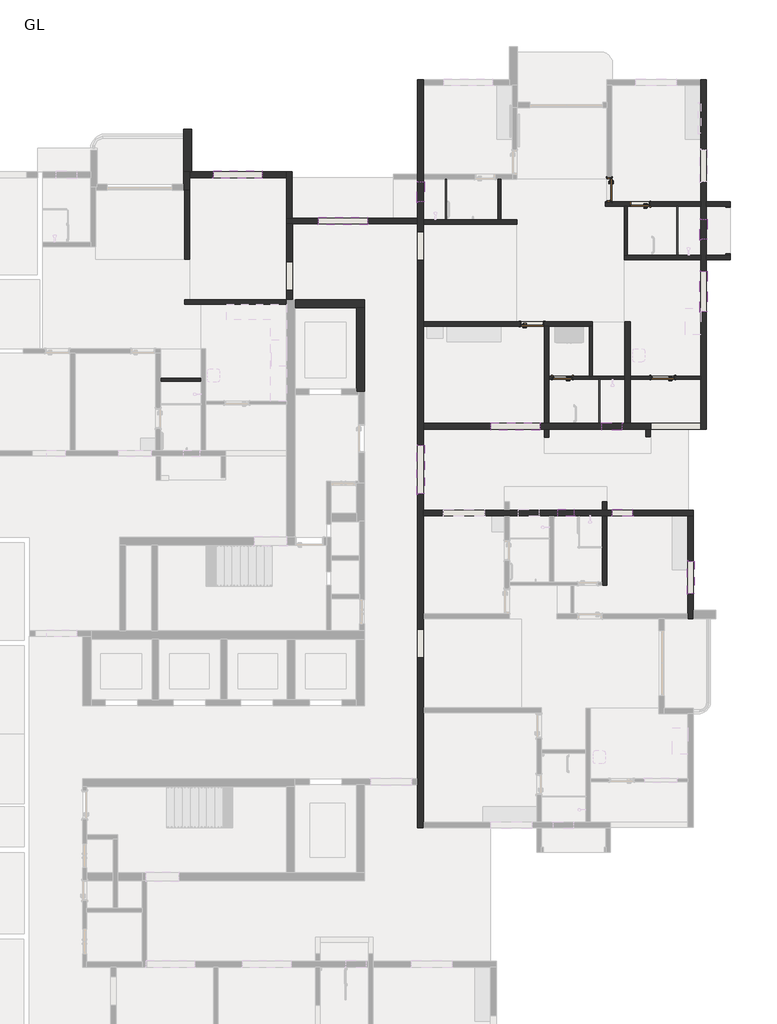
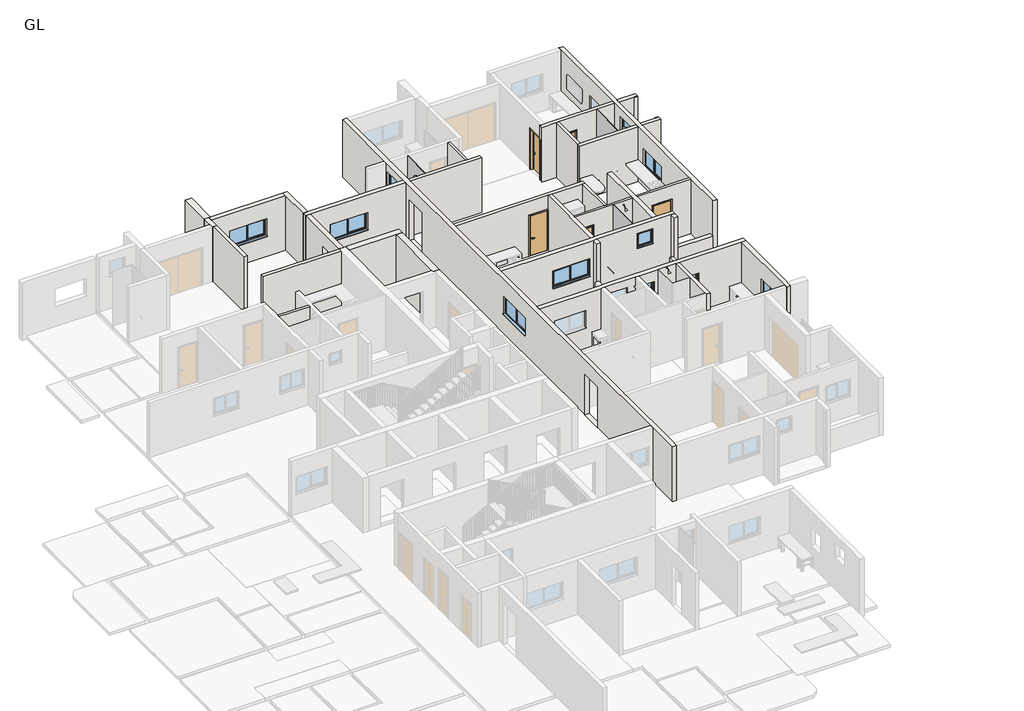
# One storey, part 6 of 14: 34 walls, 11 windows, 5 doors, 3 plates.
"""IFC4 building model written with IfcOpenShell, lengths in millimetres."""

from ifc_helpers import new_model, si_unit, origin, origin_with_axes, place, context, project, spatial, polyline, outline, extrude, faceted_brep, transform, mapped, element, save
from components import doors_intsgl_2_5_door_21b53886, doors_intsgl_2_5_door_ce04bd24, doors_intsgl_3_door_8261d8fb, doors_intsgl_3_door_f61d7fb9, doors_intsgl_3_door_77e94e6e, system_panel_glazed_1e7c63f8, system_panel_glazed_6ac8334b, system_panel_glazed_da641326, windows_dbl_plain_2_5_f94f9a84, windows_dbl_plain_4_905afcad, windows_dbl_plain_5_907a13a5, windows_dbl_plain_6_3da2432f, windows_sgl_plain_2_298b83e7, windows_sgl_plain_2_5_21186da1

model = new_model("IFC4")

# Units and contexts
model_context = context("Model", 3, world=origin())
ifc_project = project(units=[si_unit("LENGTHUNIT", "METRE", prefix="MILLI")], contexts=[model_context])

# Site, building, storey
site = spatial("IfcSite", under=ifc_project)
building = spatial("IfcBuilding", under=site)
storey = spatial("IfcBuildingStorey", under=building, Name="GL", Elevation=0.0)

# Doors
placement = place(None, origin())
doors_intsgl_2_5_door_shape = doors_intsgl_2_5_door_21b53886(model_context)
element("IfcDoor", 1, ObjectType="Doors_IntSgl : 2.5' DOOR", at=placement, inside=storey, context=model_context, shape_type="MappedRepresentation", body=[
    mapped(doors_intsgl_2_5_door_shape, transform((14743.1475488, 88467.3437403, 149.9616), x_axis=(-1.0, 0.0, 0.0), y_axis=(0.0, -1.0, 0.0), z_axis=(0.0, 0.0, 1.0))),
])
doors_intsgl_2_5_door_2_shape = doors_intsgl_2_5_door_ce04bd24(model_context)
element("IfcDoor", 2, ObjectType="Doors_IntSgl : 2.5' DOOR", at=placement, inside=storey, context=model_context, shape_type="MappedRepresentation", body=[
    mapped(doors_intsgl_2_5_door_2_shape, transform((17655.4725595, 94980.9320056, 149.9616), x_axis=(-1.0, 0.0, 0.0), y_axis=(0.0, -1.0, 0.0), z_axis=(0.0, 0.0, 1.0))),
])
doors_intsgl_3_door_shape = doors_intsgl_3_door_8261d8fb(model_context)
element("IfcDoor", 3, ObjectType="Doors_IntSgl : 3' DOOR", at=placement, inside=storey, context=model_context, shape_type="MappedRepresentation", body=[
    mapped(doors_intsgl_3_door_shape, transform((13604.2115488, 90484.8048694, 149.9616), x_axis=(1.0, 0.0, 0.0), y_axis=(0.0, 1.0, 0.0), z_axis=(0.0, 0.0, 1.0))),
])
doors_intsgl_3_door_2_shape = doors_intsgl_3_door_f61d7fb9(model_context)
element("IfcDoor", 4, ObjectType="Doors_IntSgl : 3' DOOR", at=placement, inside=storey, context=model_context, shape_type="MappedRepresentation", body=[
    mapped(doors_intsgl_3_door_2_shape, transform((16503.5076703, 95525.0000056, 149.9616), x_axis=(0.0, -1.0, 0.0), y_axis=(1.0, 0.0, 0.0), z_axis=(0.0, 0.0, 1.0))),
])
doors_intsgl_3_door_3_shape = doors_intsgl_3_door_77e94e6e(model_context)
element("IfcDoor", 5, ObjectType="Doors_IntSgl : 3' DOOR", at=placement, inside=storey, context=model_context, shape_type="MappedRepresentation", body=[
    mapped(doors_intsgl_3_door_3_shape, transform((18512.1396703, 88467.3437403, 149.9616), x_axis=(-1.0, 0.0, 0.0), y_axis=(0.0, -1.0, 0.0), z_axis=(0.0, 0.0, 1.0))),
])

# Plates
system_panel_glazed_shape = system_panel_glazed_1e7c63f8(model_context)
element("IfcPlate", 6, ObjectType="System Panel : Glazed", at=placement, inside=storey, context=model_context, shape_type="MappedRepresentation", body=[
    mapped(system_panel_glazed_shape, transform((16166.2969726, 87590.005818, 0.0), x_axis=(0.0, 1.0, 0.0), y_axis=(-1.0, 0.0, 0.0), z_axis=(0.0, 0.0, 1.0))),
])
system_panel_glazed_2_shape = system_panel_glazed_6ac8334b(model_context)
element("IfcPlate", 7, ObjectType="System Panel : Glazed", at=placement, inside=storey, context=model_context, shape_type="MappedRepresentation", body=[
    mapped(system_panel_glazed_2_shape, transform((19020.1396703, 93980.8602696, 0.0), x_axis=(0.0, -1.0, 0.0), y_axis=(1.0, 0.0, 0.0), z_axis=(0.0, 0.0, 1.0))),
])
system_panel_glazed_3_shape = system_panel_glazed_da641326(model_context)
element("IfcPlate", 8, ObjectType="System Panel : Glazed", at=placement, inside=storey, context=model_context, shape_type="MappedRepresentation", body=[
    mapped(system_panel_glazed_3_shape, transform((10397.1569726, 95164.1635363, 0.0), x_axis=(0.0, 1.0, 0.0), y_axis=(-1.0, 0.0, 0.0), z_axis=(0.0, 0.0, 1.0))),
])

# Walls
element("IfcWall", 9, ObjectType="W2", at=placement, inside=storey, context=model_context, shape_type="Brep", body=[
    faceted_brep([(16231.9624579, 83273.9078957, 0.0), (16231.9624579, 80772.0078957, 0.0), (16231.9624579, 80657.7078957, 0.0), (16231.9624579, 80657.7078957, 3000.0), (16231.9624579, 80772.0078957, 3000.0), (16231.9624579, 83273.9078957, 3000.0), (16405.6984579, 83273.9078957, 0.0), (16405.6984579, 83273.9078957, 3000.0), (16405.6984579, 80657.7078957, 3000.0), (16405.6984579, 80657.7078957, 0.0)], [[[0, 1, 2, 3, 4, 5]], [[6, 7, 8, 9]], [[2, 1, 0, 6, 9]], [[5, 4, 3, 8, 7]], [[0, 5, 7, 6]], [[3, 2, 9, 8]]]),
])
element("IfcWall", 10, ObjectType="W2", at=placement, inside=storey, context=model_context, shape_type="Brep", body=[
    faceted_brep([(17071.2725595, 93067.6565337, 0.0), (17071.2725595, 93067.6565337, 3000.0), (17185.5725595, 93067.6565337, 3000.0), (19934.5396703, 93067.6565337, 3000.0), (19934.5396703, 93067.6565337, 0.0), (17185.5725595, 93067.6565337, 0.0), (17071.2725595, 92893.9205337, 3000.0), (17071.2725595, 92893.9205337, 0.0), (19934.5396703, 92893.9205337, 0.0), (19934.5396703, 92893.9205337, 3000.0)], [[[0, 1, 2, 3, 4, 5]], [[6, 7, 8, 9]], [[7, 0, 5, 4, 8]], [[1, 6, 9, 3, 2]], [[4, 3, 9, 8]], [[1, 0, 7, 6]]]),
    faceted_brep([(21055.8975595, 93067.6565337, 3000.0), (21055.8975595, 93067.6565337, 0.0), (20882.1615595, 93067.6565337, 0.0), (20147.8996703, 93067.6565337, 0.0), (20147.8996703, 93067.6565337, 3000.0), (20882.1615595, 93067.6565337, 3000.0), (21055.8975595, 92893.9205337, 0.0), (21055.8975595, 92893.9205337, 3000.0), (20147.8996703, 92893.9205337, 3000.0), (20147.8996703, 92893.9205337, 0.0)], [[[0, 1, 2, 3, 4, 5]], [[6, 7, 8, 9]], [[1, 6, 9, 3, 2]], [[7, 0, 5, 4, 8]], [[4, 3, 9, 8]], [[1, 0, 7, 6]]]),
])
element("IfcWall", 11, ObjectType="W2", at=placement, inside=storey, context=model_context, shape_type="Brep", body=[
    faceted_brep([(16360.0725595, 95067.8000056, 0.0), (16360.0725595, 95067.8000056, 3000.0), (16416.6396703, 95067.8000056, 3000.0), (16590.3756703, 95067.8000056, 3000.0), (19934.5396703, 95067.8000056, 3000.0), (19934.5396703, 95067.8000056, 0.0), (16590.3756703, 95067.8000056, 0.0), (16416.6396703, 95067.8000056, 0.0), (17274.4725595, 95067.8000056, 2259.9616), (17274.4725595, 95067.8000056, 149.9616), (18036.4725595, 95067.8000056, 149.9616), (18036.4725595, 95067.8000056, 2259.9616), (16360.0725595, 94894.0640056, 3000.0), (16360.0725595, 94894.0640056, 0.0), (17071.2725595, 94894.0640056, 0.0), (17185.5725595, 94894.0640056, 0.0), (19934.5396703, 94894.0640056, 0.0), (19934.5396703, 94894.0640056, 3000.0), (17185.5725595, 94894.0640056, 3000.0), (17071.2725595, 94894.0640056, 3000.0), (17274.4725595, 94894.0640056, 149.9616), (17274.4725595, 94894.0640056, 2259.9616), (18036.4725595, 94894.0640056, 2259.9616), (18036.4725595, 94894.0640056, 149.9616)], [[[0, 1, 2, 3, 4, 5, 6, 7], [8, 9, 10, 11]], [[12, 13, 14, 15, 16, 17, 18, 19], [20, 21, 22, 23]], [[13, 0, 7, 6, 5, 16, 15, 14]], [[1, 0, 13, 12]], [[1, 12, 19, 18, 17, 4, 3, 2]], [[5, 4, 17, 16]], [[20, 9, 8, 21]], [[21, 8, 11, 22]], [[10, 23, 22, 11]], [[9, 20, 23, 10]]]),
    faceted_brep([(21055.8975595, 95067.8000056, 3000.0), (21055.8975595, 95067.8000056, 0.0), (20147.8996703, 95067.8000056, 0.0), (20147.8996703, 95067.8000056, 3000.0), (21055.8975595, 94894.0640056, 0.0), (21055.8975595, 94894.0640056, 3000.0), (20882.1615595, 94894.0640056, 3000.0), (20147.8996703, 94894.0640056, 3000.0), (20147.8996703, 94894.0640056, 0.0), (20882.1615595, 94894.0640056, 0.0)], [[[0, 1, 2, 3]], [[4, 5, 6, 7, 8, 9]], [[1, 4, 9, 8, 2]], [[5, 0, 3, 7, 6]], [[3, 2, 8, 7]], [[1, 0, 5, 4]]]),
])
element("IfcWall", 12, ObjectType="W2", at=placement, inside=storey, context=model_context, shape_type="SweptSolid", body=[
    extrude(outline(polyline([(20882.1615595, 94855.9640056), (20882.1615595, 94894.0640056), (21055.8975595, 94894.0640056), (21055.8975595, 94855.9640056), (20882.1615595, 94855.9640056)])), origin_with_axes(), (0.0, 0.0, 1.0), 3000.0),
])
element("IfcWall", 13, ObjectType="W2", at=placement, inside=storey, context=model_context, shape_type="SweptSolid", body=[
    extrude(outline(polyline([(20882.1615595, 93067.6565337), (20882.1615595, 93112.1065337), (21055.8975595, 93112.1065337), (21055.8975595, 93067.6565337), (20882.1615595, 93067.6565337)])), origin_with_axes(), (0.0, 0.0, 1.0), 3000.0),
])
element("IfcWall", 14, ObjectType="W2", at=placement, inside=storey, context=model_context, shape_type="Brep", body=[
    faceted_brep([(13025.3335039, 94403.2709831, 0.0), (12427.5760982, 94403.2709831, 0.0), (12313.2760982, 94403.2709831, 0.0), (9508.1569726, 94403.2709831, 0.0), (9508.1569726, 94403.2709831, 3000.0), (12313.2760982, 94403.2709831, 3000.0), (12427.5760982, 94403.2709831, 3000.0), (13025.3335039, 94403.2709831, 3000.0), (13025.3335039, 94229.5349831, 0.0), (13025.3335039, 94229.5349831, 3000.0), (9508.1569726, 94229.5349831, 3000.0), (9508.1569726, 94229.5349831, 0.0)], [[[0, 1, 2, 3, 4, 5, 6, 7]], [[8, 9, 10, 11]], [[3, 2, 1, 0, 8, 11]], [[7, 6, 5, 4, 10, 9]], [[0, 7, 9, 8]], [[4, 3, 11, 10]]]),
])
element("IfcWall", 15, ObjectType="W2", at=placement, inside=storey, context=model_context, shape_type="Brep", body=[
    faceted_brep([(9508.1569726, 90397.9368694, 0.0), (14061.4115488, 90397.9368694, 0.0), (14235.1475488, 90397.9368694, 0.0), (15750.2069726, 90397.9368694, 0.0), (15864.5069726, 90397.9368694, 0.0), (15864.5069726, 90397.9368694, 3000.0), (15750.2069726, 90397.9368694, 3000.0), (14235.1475488, 90397.9368694, 3000.0), (14061.4115488, 90397.9368694, 3000.0), (9508.1569726, 90397.9368694, 3000.0), (14061.4115488, 90397.9368694, 2259.9616), (14061.4115488, 90397.9368694, 149.9616), (13147.0115488, 90397.9368694, 149.9616), (13147.0115488, 90397.9368694, 2259.9616), (15864.5069726, 90571.6728694, 0.0), (9508.1569726, 90571.6728694, 0.0), (9508.1569726, 90571.6728694, 3000.0), (15864.5069726, 90571.6728694, 3000.0), (14061.4115488, 90571.6728694, 149.9616), (14061.4115488, 90571.6728694, 2259.9616), (13147.0115488, 90571.6728694, 2259.9616), (13147.0115488, 90571.6728694, 149.9616)], [[[0, 1, 2, 3, 4, 5, 6, 7, 8, 9], [10, 11, 12, 13]], [[14, 15, 16, 17], [18, 19, 20, 21]], [[4, 3, 2, 1, 0, 15, 14]], [[9, 8, 7, 6, 5, 17, 16]], [[0, 9, 16, 15]], [[5, 4, 14, 17]], [[18, 11, 10, 19]], [[19, 10, 13, 20]], [[20, 13, 12, 21]], [[11, 18, 21, 12]]]),
])
element("IfcWall", 16, ObjectType="W2", at=placement, inside=storey, context=model_context, shape_type="Brep", body=[
    faceted_brep([(14061.4115488, 90397.9368694, 0.0), (14061.4115488, 86744.8178957, 0.0), (14061.4115488, 86744.8178957, 3000.0), (14061.4115488, 90397.9368694, 3000.0), (14235.1475488, 90397.9368694, 0.0), (14235.1475488, 90397.9368694, 3000.0), (14235.1475488, 88524.4937403, 3000.0), (14235.1475488, 88410.1937403, 3000.0), (14235.1475488, 86744.8178957, 3000.0), (14235.1475488, 86744.8178957, 0.0), (14235.1475488, 88410.1937403, 0.0), (14235.1475488, 88524.4937403, 0.0)], [[[0, 1, 2, 3]], [[4, 5, 6, 7, 8, 9, 10, 11]], [[1, 0, 4, 11, 10, 9]], [[3, 2, 8, 7, 6, 5]], [[0, 3, 5, 4]], [[2, 1, 9, 8]]]),
])
element("IfcWall", 17, ObjectType="W2", at=placement, inside=storey, context=model_context, shape_type="SweptSolid", body=[
    extrude(outline(polyline([(14061.4115488, 86232.3368694), (14061.4115488, 86531.4578957), (14235.1475488, 86531.4578957), (14235.1475488, 86232.3368694), (14061.4115488, 86232.3368694)])), origin_with_axes(), (0.0, 0.0, 1.0), 3000.0),
])
element("IfcWall", 18, ObjectType="W2", at=placement, inside=storey, context=model_context, shape_type="SweptSolid", body=[
    extrude(outline(polyline([(541.6073716, 92913.0456254), (541.6073716, 95510.1956254), (715.3433716, 95510.1956254), (715.3433716, 92913.0456254), (541.6073716, 92913.0456254)])), origin_with_axes(), (0.0, 0.0, 1.0), 3000.0),
])
element("IfcWall", 19, ObjectType="W2", at=placement, inside=storey, context=model_context, shape_type="Brep", body=[
    faceted_brep([(4376.8368387, 91396.9573985, 0.0), (4369.7369726, 91396.9573985, 0.0), (540.6869726, 91396.9573985, 0.0), (540.6869726, 91396.9573985, 3000.0), (4369.7369726, 91396.9573985, 3000.0), (4376.8368387, 91396.9573985, 3000.0), (4376.8368387, 91223.2213985, 0.0), (4376.8368387, 91223.2213985, 3000.0), (540.6869726, 91223.2213985, 3000.0), (540.6869726, 91223.2213985, 0.0)], [[[0, 1, 2, 3, 4, 5]], [[6, 7, 8, 9]], [[2, 1, 0, 6, 9]], [[3, 2, 9, 8]], [[5, 4, 3, 8, 7]], [[0, 5, 7, 6]]]),
])
element("IfcWall", 20, ObjectType="W2", at=placement, inside=storey, context=model_context, shape_type="SweptSolid", body=[
    extrude(outline(polyline([(16405.6984579, 83792.0678957), (16405.6984579, 83487.2678957), (16231.9624579, 83487.2678957), (16231.9624579, 83792.0678957), (16405.6984579, 83792.0678957)])), origin_with_axes(), (0.0, 0.0, 1.0), 3000.0),
])
element("IfcWall", 21, ObjectType="W2", at=placement, inside=storey, context=model_context, shape_type="SweptSolid", body=[
    extrude(outline(polyline([(14061.4115488, 86232.3368694), (14061.4115488, 86531.4578957), (14235.1475488, 86531.4578957), (14235.1475488, 86232.3368694), (14061.4115488, 86232.3368694)])), origin_with_axes(), (0.0, 0.0, 1.0), 3000.0),
])
element("IfcWall", 22, ObjectType="W2", at=placement, inside=storey, context=model_context, shape_type="SweptSolid", body=[
    extrude(outline(polyline([(17877.4569726, 86252.0578957), (17877.4569726, 86531.4578957), (18051.1929726, 86531.4578957), (18051.1929726, 86252.0578957), (17877.4569726, 86252.0578957)])), origin_with_axes(), (0.0, 0.0, 1.0), 3000.0),
])
element("IfcWall", 23, ObjectType="W3", at=placement, inside=storey, context=model_context, shape_type="SweptSolid", body=[
    extrude(outline(polyline([(17071.2725595, 93067.6565337), (17071.2725595, 94894.0640056), (17185.5725595, 94894.0640056), (17185.5725595, 93067.6565337), (17071.2725595, 93067.6565337)])), origin_with_axes(), (0.0, 0.0, 1.0), 3000.0),
])
element("IfcWall", 24, ObjectType="W3", at=placement, inside=storey, context=model_context, shape_type="SweptSolid", body=[
    extrude(outline(polyline([(12313.2760982, 94403.2709831), (12313.2760982, 95925.0560895), (12427.5760982, 95925.0560895), (12427.5760982, 94403.2709831), (12313.2760982, 94403.2709831)])), origin_with_axes(), (0.0, 0.0, 1.0), 3000.0),
])
element("IfcWall", 25, ObjectType="W3", at=placement, inside=storey, context=model_context, shape_type="SweptSolid", body=[
    extrude(outline(polyline([(15750.2069726, 88524.4937403), (15750.2069726, 90397.9368694), (15864.5069726, 90397.9368694), (15864.5069726, 88524.4937403), (15750.2069726, 88524.4937403)])), origin_with_axes(), (0.0, 0.0, 1.0), 3000.0),
])
element("IfcWall", 26, ObjectType="W3", at=placement, inside=storey, context=model_context, shape_type="Brep", body=[
    faceted_brep([(19934.5396703, 88524.4937403, 3000.0), (19934.5396703, 88524.4937403, 0.0), (17293.2569726, 88524.4937403, 0.0), (17293.2569726, 88524.4937403, 3000.0), (18054.9396703, 88524.4937403, 2259.9616), (18054.9396703, 88524.4937403, 149.9616), (18969.3396703, 88524.4937403, 149.9616), (18969.3396703, 88524.4937403, 2259.9616), (19934.5396703, 88410.1937403, 0.0), (19934.5396703, 88410.1937403, 3000.0), (17293.2569726, 88410.1937403, 3000.0), (17293.2569726, 88410.1937403, 0.0), (18054.9396703, 88410.1937403, 149.9616), (18054.9396703, 88410.1937403, 2259.9616), (18969.3396703, 88410.1937403, 2259.9616), (18969.3396703, 88410.1937403, 149.9616)], [[[0, 1, 2, 3], [4, 5, 6, 7]], [[8, 9, 10, 11], [12, 13, 14, 15]], [[1, 8, 11, 2]], [[9, 0, 3, 10]], [[1, 0, 9, 8]], [[3, 2, 11, 10]], [[12, 5, 4, 13]], [[13, 4, 7, 14]], [[6, 15, 14, 7]], [[5, 12, 15, 6]]]),
    faceted_brep([(14235.1475488, 88524.4937403, 0.0), (14235.1475488, 88524.4937403, 3000.0), (15750.2069726, 88524.4937403, 3000.0), (15864.5069726, 88524.4937403, 3000.0), (17079.8969726, 88524.4937403, 3000.0), (17079.8969726, 88524.4937403, 0.0), (15864.5069726, 88524.4937403, 0.0), (15750.2069726, 88524.4937403, 0.0), (14362.1475488, 88524.4937403, 2259.9616), (14362.1475488, 88524.4937403, 149.9616), (15124.1475488, 88524.4937403, 149.9616), (15124.1475488, 88524.4937403, 2259.9616), (14235.1475488, 88410.1937403, 3000.0), (14235.1475488, 88410.1937403, 0.0), (17079.8969726, 88410.1937403, 0.0), (17079.8969726, 88410.1937403, 3000.0), (14362.1475488, 88410.1937403, 149.9616), (14362.1475488, 88410.1937403, 2259.9616), (15124.1475488, 88410.1937403, 2259.9616), (15124.1475488, 88410.1937403, 149.9616)], [[[0, 1, 2, 3, 4, 5, 6, 7], [8, 9, 10, 11]], [[12, 13, 14, 15], [16, 17, 18, 19]], [[13, 0, 7, 6, 5, 14]], [[1, 12, 15, 4, 3, 2]], [[5, 4, 15, 14]], [[1, 0, 13, 12]], [[16, 9, 8, 17]], [[17, 8, 11, 18]], [[10, 19, 18, 11]], [[9, 16, 19, 10]]]),
])
element("IfcWall", 27, ObjectType="W3", at=placement, inside=storey, context=model_context, shape_type="SweptSolid", body=[
    extrude(outline(polyline([(-371.094999, 88436.0416254), (1156.969001, 88436.0416254), (1156.969001, 88321.7416254), (-371.094999, 88321.7416254), (-371.094999, 88436.0416254)])), origin_with_axes(), (0.0, 0.0, 1.0), 3000.0),
])
element("IfcWall", 28, ObjectType="W4", at=placement, inside=storey, context=model_context, shape_type="Brep", body=[
    faceted_brep([(501.9833716, 97794.9636787, 0.0), (501.9833716, 96193.9709831, 0.0), (501.9833716, 96193.9709831, 3000.0), (501.9833716, 97794.9636787, 3000.0), (806.7833716, 97794.9636787, 0.0), (806.7833716, 97794.9636787, 3000.0), (806.7833716, 96193.9709831, 3000.0), (806.7833716, 96193.9709831, 0.0), (715.3433716, 96193.9709831, 0.0), (715.3433716, 96193.9709831, 3000.0)], [[[0, 1, 2, 3]], [[4, 5, 6, 7]], [[1, 0, 4, 7, 8]], [[3, 2, 9, 6, 5]], [[0, 3, 5, 4]], [[2, 1, 8, 7, 6, 9]]]),
])
element("IfcWall", 29, ObjectType="W4", at=placement, inside=storey, context=model_context, shape_type="Brep", body=[
    faceted_brep([(4681.6368387, 91092.1573985, 0.0), (6993.0368387, 91092.1573985, 0.0), (7297.8368387, 91092.1573985, 0.0), (7297.8368387, 91092.1573985, 3000.0), (6993.0368387, 91092.1573985, 3000.0), (4681.6368387, 91092.1573985, 3000.0), (4681.6368387, 91396.9573985, 0.0), (4681.6368387, 91396.9573985, 3000.0), (7297.8368387, 91396.9573985, 3000.0), (7297.8368387, 91396.9573985, 0.0)], [[[0, 1, 2, 3, 4, 5]], [[6, 7, 8, 9]], [[2, 1, 0, 6, 9]], [[5, 4, 3, 8, 7]], [[0, 5, 7, 6]], [[3, 2, 9, 8]]]),
])
element("IfcWall", 30, ObjectType="W4", at=placement, inside=storey, context=model_context, shape_type="Brep", body=[
    faceted_brep([(6993.0368387, 91092.1573985, 0.0), (6993.0368387, 88039.0502935, 0.0), (6993.0368387, 87927.7982935, 0.0), (6993.0368387, 87927.7982935, 3000.0), (6993.0368387, 88039.0502935, 3000.0), (6993.0368387, 91092.1573985, 3000.0), (7297.8368387, 91092.1573985, 0.0), (7297.8368387, 91092.1573985, 3000.0), (7297.8368387, 87927.7982935, 3000.0), (7297.8368387, 87927.7982935, 0.0), (7297.3568654, 87927.7982935, 0.0), (7068.7568654, 87927.7982935, 0.0), (7297.3568654, 87927.7982935, 3000.0), (7068.7568654, 87927.7982935, 3000.0)], [[[0, 1, 2, 3, 4, 5]], [[6, 7, 8, 9]], [[2, 1, 0, 6, 9, 10, 11]], [[3, 2, 11, 10, 9, 8, 12, 13]], [[5, 4, 3, 13, 12, 8, 7]], [[0, 5, 7, 6]]]),
])
element("IfcWall", 31, ObjectType="W7", at=placement, inside=storey, context=model_context, shape_type="Brep", body=[
    faceted_brep([(4369.7369726, 94240.7109831, 0.0), (4369.7369726, 91396.9573985, 0.0), (4369.7369726, 91396.9573985, 3000.0), (4369.7369726, 94240.7109831, 3000.0), (4369.7369726, 92819.3573985, 2259.9616), (4369.7369726, 91752.5573985, 2259.9616), (4369.7369726, 91752.5573985, 149.9616), (4369.7369726, 92819.3573985, 149.9616), (4592.2409726, 94240.7109831, 0.0), (4592.2409726, 94240.7109831, 3000.0), (4592.2409726, 91396.9573985, 3000.0), (4592.2409726, 91396.9573985, 0.0), (4592.2409726, 92819.3573985, 2259.9616), (4592.2409726, 92819.3573985, 149.9616), (4592.2409726, 91752.5573985, 149.9616), (4592.2409726, 91752.5573985, 2259.9616), (4376.8368387, 91396.9573985, 0.0), (4376.8368387, 91396.9573985, 3000.0)], [[[0, 1, 2, 3], [4, 5, 6, 7]], [[8, 9, 10, 11], [12, 13, 14, 15]], [[1, 0, 8, 11, 16]], [[3, 2, 17, 10, 9]], [[0, 3, 9, 8]], [[2, 1, 16, 11, 10, 17]], [[13, 12, 4, 7]], [[14, 13, 7, 6]], [[15, 14, 6, 5]], [[12, 15, 5, 4]]]),
])
element("IfcWall", 32, ObjectType="W8", at=placement, inside=storey, context=model_context, shape_type="Brep", body=[
    faceted_brep([(9508.1569726, 71549.2678957, 0.0), (9508.1569726, 71762.6278957, 0.0), (9508.1569726, 75881.5131416, 0.0), (9508.1569726, 76055.2491416, 0.0), (9508.1569726, 79413.1078957, 0.0), (9508.1569726, 79586.8438957, 0.0), (9508.1569726, 83273.9078957, 0.0), (9508.1569726, 83487.2678957, 0.0), (9508.1569726, 86531.4578957, 0.0), (9508.1569726, 86744.8178957, 0.0), (9508.1569726, 90397.9368694, 0.0), (9508.1569726, 90571.6728694, 0.0), (9508.1569726, 94229.5349831, 0.0), (9508.1569726, 94403.2709831, 0.0), (9508.1569726, 95925.0560895, 0.0), (9508.1569726, 96098.7920895, 0.0), (9508.1569726, 99449.8978957, 0.0), (9508.1569726, 99648.0178957, 0.0), (9508.1569726, 99648.0178957, 3000.0), (9508.1569726, 99449.8978957, 3000.0), (9508.1569726, 96098.7920895, 3000.0), (9508.1569726, 95925.0560895, 3000.0), (9508.1569726, 94403.2709831, 3000.0), (9508.1569726, 94229.5349831, 3000.0), (9508.1569726, 90571.6728694, 3000.0), (9508.1569726, 90397.9368694, 3000.0), (9508.1569726, 86744.8178957, 3000.0), (9508.1569726, 86531.4578957, 3000.0), (9508.1569726, 83487.2678957, 3000.0), (9508.1569726, 83273.9078957, 3000.0), (9508.1569726, 79586.8438957, 3000.0), (9508.1569726, 79413.1078957, 3000.0), (9508.1569726, 76055.2491416, 3000.0), (9508.1569726, 75881.5131416, 3000.0), (9508.1569726, 71762.6278957, 3000.0), (9508.1569726, 71549.2678957, 3000.0), (9508.1569726, 85923.7628957, 2110.0), (9508.1569726, 85923.7628957, 1200.0), (9508.1569726, 84094.9628957, 1200.0), (9508.1569726, 84094.9628957, 2110.0), (9508.1569726, 95825.6709831, 2590.8), (9508.1569726, 95825.6709831, 1828.8), (9508.1569726, 95063.6709831, 1828.8), (9508.1569726, 95063.6709831, 2590.8), (9508.1569726, 77939.9078957, 2259.9616), (9508.1569726, 79006.7078957, 2259.9616), (9508.1569726, 79006.7078957, 149.9616), (9508.1569726, 77939.9078957, 149.9616), (9508.1569726, 92883.3349831, 2259.9616), (9508.1569726, 93950.1349831, 2259.9616), (9508.1569726, 93950.1349831, 149.9616), (9508.1569726, 92883.3349831, 149.9616), (9294.7969726, 71549.2678957, 0.0), (9294.7969726, 71549.2678957, 3000.0), (9294.7969726, 73177.9138911, 3000.0), (9294.7969726, 73400.4178911, 3000.0), (9294.7969726, 94240.7109831, 3000.0), (9294.7969726, 94454.0709831, 3000.0), (9294.7969726, 95925.0560895, 3000.0), (9294.7969726, 96098.7920895, 3000.0), (9294.7969726, 99648.0178957, 3000.0), (9294.7969726, 99648.0178957, 0.0), (9294.7969726, 96098.7920895, 0.0), (9294.7969726, 95925.0560895, 0.0), (9294.7969726, 94454.0709831, 0.0), (9294.7969726, 94240.7109831, 0.0), (9294.7969726, 73400.4178911, 0.0), (9294.7969726, 73177.9138911, 0.0), (9294.7969726, 85923.7628957, 2110.0), (9294.7969726, 84094.9628957, 2110.0), (9294.7969726, 84094.9628957, 1200.0), (9294.7969726, 85923.7628957, 1200.0), (9294.7969726, 95825.6709831, 2590.8), (9294.7969726, 95063.6709831, 2590.8), (9294.7969726, 95063.6709831, 1828.8), (9294.7969726, 95825.6709831, 1828.8), (9294.7969726, 77939.9078957, 2259.9616), (9294.7969726, 77939.9078957, 149.9616), (9294.7969726, 79006.7078957, 149.9616), (9294.7969726, 79006.7078957, 2259.9616), (9294.7969726, 92883.3349831, 2259.9616), (9294.7969726, 92883.3349831, 149.9616), (9294.7969726, 93950.1349831, 149.9616), (9294.7969726, 93950.1349831, 2259.9616)], [[[0, 1, 2, 3, 4, 5, 6, 7, 8, 9, 10, 11, 12, 13, 14, 15, 16, 17, 18, 19, 20, 21, 22, 23, 24, 25, 26, 27, 28, 29, 30, 31, 32, 33, 34, 35], [36, 37, 38, 39], [40, 41, 42, 43], [44, 45, 46, 47], [48, 49, 50, 51]], [[52, 53, 54, 55, 56, 57, 58, 59, 60, 61, 62, 63, 64, 65, 66, 67], [68, 69, 70, 71], [72, 73, 74, 75], [76, 77, 78, 79], [80, 81, 82, 83]], [[17, 16, 15, 14, 13, 12, 11, 10, 9, 8, 7, 6, 5, 4, 3, 2, 1, 0, 52, 67, 66, 65, 64, 63, 62, 61]], [[35, 34, 33, 32, 31, 30, 29, 28, 27, 26, 25, 24, 23, 22, 21, 20, 19, 18, 60, 59, 58, 57, 56, 55, 54, 53]], [[0, 35, 53, 52]], [[18, 17, 61, 60]], [[37, 36, 68, 71]], [[38, 37, 71, 70]], [[39, 38, 70, 69]], [[36, 39, 69, 68]], [[41, 40, 72, 75]], [[42, 41, 75, 74]], [[43, 42, 74, 73]], [[40, 43, 73, 72]], [[77, 76, 44, 47]], [[78, 77, 47, 46]], [[79, 78, 46, 45]], [[76, 79, 45, 44]], [[81, 80, 48, 51]], [[82, 81, 51, 50]], [[83, 82, 50, 49]], [[80, 83, 49, 48]]]),
])
element("IfcWall", 33, ObjectType="W8", at=placement, inside=storey, context=model_context, shape_type="Brep", body=[
    faceted_brep([(9508.1569726, 83273.9078957, 0.0), (12563.4404579, 83273.9078957, 0.0), (12737.1764579, 83273.9078957, 0.0), (14242.1264579, 83273.9078957, 0.0), (14415.8624579, 83273.9078957, 0.0), (16231.9624579, 83273.9078957, 0.0), (16405.6984579, 83273.9078957, 0.0), (19454.7969726, 83273.9078957, 0.0), (19668.1569726, 83273.9078957, 0.0), (19668.1569726, 83273.9078957, 3000.0), (19454.7969726, 83273.9078957, 3000.0), (16405.6984579, 83273.9078957, 3000.0), (16231.9624579, 83273.9078957, 3000.0), (14415.8624579, 83273.9078957, 3000.0), (14242.1264579, 83273.9078957, 3000.0), (12737.1764579, 83273.9078957, 3000.0), (12563.4404579, 83273.9078957, 3000.0), (9508.1569726, 83273.9078957, 3000.0), (16608.8984579, 83273.9078957, 2110.0), (17370.8984579, 83273.9078957, 2110.0), (17370.8984579, 83273.9078957, 1200.0), (16608.8984579, 83273.9078957, 1200.0), (14568.2624579, 83273.9078957, 2438.4), (15177.8624579, 83273.9078957, 2438.4), (15177.8624579, 83273.9078957, 1828.8), (14568.2624579, 83273.9078957, 1828.8), (13092.7764579, 83273.9078957, 2590.8), (13854.7764579, 83273.9078957, 2590.8), (13854.7764579, 83273.9078957, 1828.8), (13092.7764579, 83273.9078957, 1828.8), (10273.7987153, 83273.9078957, 2110.0), (11797.7987153, 83273.9078957, 2110.0), (11797.7987153, 83273.9078957, 1200.0), (10273.7987153, 83273.9078957, 1200.0), (9508.1569726, 83487.2678957, 0.0), (9508.1569726, 83487.2678957, 3000.0), (12563.4404579, 83487.2678957, 3000.0), (12737.1764579, 83487.2678957, 3000.0), (16231.9624579, 83487.2678957, 3000.0), (16405.6984579, 83487.2678957, 3000.0), (19668.1569726, 83487.2678957, 3000.0), (19668.1569726, 83487.2678957, 0.0), (16405.6984579, 83487.2678957, 0.0), (16231.9624579, 83487.2678957, 0.0), (12737.1764579, 83487.2678957, 0.0), (12563.4404579, 83487.2678957, 0.0), (16608.8984579, 83487.2678957, 2110.0), (16608.8984579, 83487.2678957, 1200.0), (17370.8984579, 83487.2678957, 1200.0), (17370.8984579, 83487.2678957, 2110.0), (14568.2624579, 83487.2678957, 2438.4), (14568.2624579, 83487.2678957, 1828.8), (15177.8624579, 83487.2678957, 1828.8), (15177.8624579, 83487.2678957, 2438.4), (13092.7764579, 83487.2678957, 2590.8), (13092.7764579, 83487.2678957, 1828.8), (13854.7764579, 83487.2678957, 1828.8), (13854.7764579, 83487.2678957, 2590.8), (10273.7987153, 83487.2678957, 2110.0), (10273.7987153, 83487.2678957, 1200.0), (11797.7987153, 83487.2678957, 1200.0), (11797.7987153, 83487.2678957, 2110.0)], [[[0, 1, 2, 3, 4, 5, 6, 7, 8, 9, 10, 11, 12, 13, 14, 15, 16, 17], [18, 19, 20, 21], [22, 23, 24, 25], [26, 27, 28, 29], [30, 31, 32, 33]], [[34, 35, 36, 37, 38, 39, 40, 41, 42, 43, 44, 45], [46, 47, 48, 49], [50, 51, 52, 53], [54, 55, 56, 57], [58, 59, 60, 61]], [[8, 7, 6, 5, 4, 3, 2, 1, 0, 34, 45, 44, 43, 42, 41]], [[17, 16, 15, 14, 13, 12, 11, 10, 9, 40, 39, 38, 37, 36, 35]], [[0, 17, 35, 34]], [[9, 8, 41, 40]], [[47, 46, 18, 21]], [[48, 47, 21, 20]], [[49, 48, 20, 19]], [[46, 49, 19, 18]], [[51, 50, 22, 25]], [[52, 51, 25, 24]], [[53, 52, 24, 23]], [[50, 53, 23, 22]], [[55, 54, 26, 29]], [[56, 55, 29, 28]], [[57, 56, 28, 27]], [[54, 57, 27, 26]], [[59, 58, 30, 33]], [[60, 59, 33, 32]], [[61, 60, 32, 31]], [[58, 61, 31, 30]]]),
])
element("IfcWall", 34, ObjectType="W8", at=placement, inside=storey, context=model_context, shape_type="Brep", body=[
    faceted_brep([(19454.7969726, 83273.9078957, 0.0), (19454.7969726, 79586.8438957, 0.0), (19454.7969726, 79413.1078957, 0.0), (19454.7969726, 79413.1078957, 3000.0), (19454.7969726, 79586.8438957, 3000.0), (19454.7969726, 83273.9078957, 3000.0), (19454.7969726, 81572.1078957, 2110.0), (19454.7969726, 80352.9078957, 2110.0), (19454.7969726, 80352.9078957, 1200.0), (19454.7969726, 81572.1078957, 1200.0), (19668.1569726, 83273.9078957, 0.0), (19668.1569726, 83273.9078957, 3000.0), (19668.1569726, 79717.9078957, 3000.0), (19668.1569726, 79413.1078957, 3000.0), (19668.1569726, 79413.1078957, 0.0), (19668.1569726, 79717.9078957, 0.0), (19668.1569726, 81572.1078957, 2110.0), (19668.1569726, 81572.1078957, 1200.0), (19668.1569726, 80352.9078957, 1200.0), (19668.1569726, 80352.9078957, 2110.0)], [[[0, 1, 2, 3, 4, 5], [6, 7, 8, 9]], [[10, 11, 12, 13, 14, 15], [16, 17, 18, 19]], [[2, 1, 0, 10, 15, 14]], [[5, 4, 3, 13, 12, 11]], [[0, 5, 11, 10]], [[3, 2, 14, 13]], [[17, 16, 6, 9]], [[18, 17, 9, 8]], [[19, 18, 8, 7]], [[16, 19, 7, 6]]]),
])
element("IfcWall", 35, ObjectType="W8", at=placement, inside=storey, context=model_context, shape_type="Brep", body=[
    faceted_brep([(9508.1569726, 86531.4578957, 0.0), (14061.4115488, 86531.4578957, 0.0), (14235.1475488, 86531.4578957, 0.0), (17877.4569726, 86531.4578957, 0.0), (18051.1929726, 86531.4578957, 0.0), (18054.9396703, 86531.4578957, 0.0), (18054.9396703, 86531.4578957, 1171.2), (18054.9396703, 86531.4578957, 3000.0), (18051.1929726, 86531.4578957, 3000.0), (17877.4569726, 86531.4578957, 3000.0), (14235.1475488, 86531.4578957, 3000.0), (14061.4115488, 86531.4578957, 3000.0), (9508.1569726, 86531.4578957, 3000.0), (13883.6115488, 86531.4578957, 2110.0), (13883.6115488, 86531.4578957, 1200.0), (12054.8115488, 86531.4578957, 1200.0), (12054.8115488, 86531.4578957, 2110.0), (16978.2969726, 86531.4578957, 2590.8), (16978.2969726, 86531.4578957, 1828.8), (16216.2969726, 86531.4578957, 1828.8), (16216.2969726, 86531.4578957, 2590.8), (9508.1569726, 86744.8178957, 0.0), (9508.1569726, 86744.8178957, 3000.0), (14061.4115488, 86744.8178957, 3000.0), (14235.1475488, 86744.8178957, 3000.0), (17079.8969726, 86744.8178957, 3000.0), (17293.2569726, 86744.8178957, 3000.0), (18054.9396703, 86744.8178957, 3000.0), (18054.9396703, 86744.8178957, 1171.2), (18054.9396703, 86744.8178957, 0.0), (17293.2569726, 86744.8178957, 0.0), (17079.8969726, 86744.8178957, 0.0), (14235.1475488, 86744.8178957, 0.0), (14061.4115488, 86744.8178957, 0.0), (13883.6115488, 86744.8178957, 2110.0), (12054.8115488, 86744.8178957, 2110.0), (12054.8115488, 86744.8178957, 1200.0), (13883.6115488, 86744.8178957, 1200.0), (16978.2969726, 86744.8178957, 2590.8), (16216.2969726, 86744.8178957, 2590.8), (16216.2969726, 86744.8178957, 1828.8), (16978.2969726, 86744.8178957, 1828.8)], [[[0, 1, 2, 3, 4, 5, 6, 7, 8, 9, 10, 11, 12], [13, 14, 15, 16], [17, 18, 19, 20]], [[21, 22, 23, 24, 25, 26, 27, 28, 29, 30, 31, 32, 33], [34, 35, 36, 37], [38, 39, 40, 41]], [[5, 4, 3, 2, 1, 0, 21, 33, 32, 31, 30, 29]], [[7, 6, 5, 29, 28, 27]], [[12, 11, 10, 9, 8, 7, 27, 26, 25, 24, 23, 22]], [[0, 12, 22, 21]], [[14, 13, 34, 37]], [[15, 14, 37, 36]], [[16, 15, 36, 35]], [[13, 16, 35, 34]], [[18, 17, 38, 41]], [[19, 18, 41, 40]], [[20, 19, 40, 39]], [[17, 20, 39, 38]]]),
])
element("IfcWall", 36, ObjectType="W8", at=placement, inside=storey, context=model_context, shape_type="Brep", body=[
    faceted_brep([(17293.2569726, 86744.8178957, 0.0), (17293.2569726, 88410.1937403, 0.0), (17293.2569726, 88524.4937403, 0.0), (17293.2569726, 90568.7878957, 0.0), (17293.2569726, 90568.7878957, 3000.0), (17293.2569726, 88524.4937403, 3000.0), (17293.2569726, 88410.1937403, 3000.0), (17293.2569726, 86744.8178957, 3000.0), (17079.8969726, 86744.8178957, 0.0), (17079.8969726, 86744.8178957, 3000.0), (17079.8969726, 88410.1937403, 3000.0), (17079.8969726, 88524.4937403, 3000.0), (17079.8969726, 90568.7878957, 3000.0), (17079.8969726, 90568.7878957, 0.0), (17079.8969726, 88524.4937403, 0.0), (17079.8969726, 88410.1937403, 0.0)], [[[0, 1, 2, 3, 4, 5, 6, 7]], [[8, 9, 10, 11, 12, 13, 14, 15]], [[3, 2, 1, 0, 8, 15, 14, 13]], [[4, 3, 13, 12]], [[7, 6, 5, 4, 12, 11, 10, 9]], [[0, 7, 9, 8]]]),
])
element("IfcWall", 37, ObjectType="W8", at=placement, inside=storey, context=model_context, shape_type="Brep", body=[
    faceted_brep([(20147.8996703, 86531.4578957, 0.0), (20147.8996703, 92893.9205337, 0.0), (20147.8996703, 93067.6565337, 0.0), (20147.8996703, 94894.0640056, 0.0), (20147.8996703, 95067.8000056, 0.0), (20147.8996703, 99650.9820895, 0.0), (20147.8996703, 99650.9820895, 3000.0), (20147.8996703, 95067.8000056, 3000.0), (20147.8996703, 94894.0640056, 3000.0), (20147.8996703, 93067.6565337, 3000.0), (20147.8996703, 92893.9205337, 3000.0), (20147.8996703, 86531.4578957, 3000.0), (20147.8996703, 92461.4937403, 2110.0), (20147.8996703, 92461.4937403, 1200.0), (20147.8996703, 90937.4937403, 1200.0), (20147.8996703, 90937.4937403, 2110.0), (20147.8996703, 94417.2937403, 2590.8), (20147.8996703, 94417.2937403, 1828.8), (20147.8996703, 93655.2937403, 1828.8), (20147.8996703, 93655.2937403, 2590.8), (20147.8996703, 97033.4937403, 2110.0), (20147.8996703, 97033.4937403, 1200.0), (20147.8996703, 95814.2937403, 1200.0), (20147.8996703, 95814.2937403, 2110.0), (19934.5396703, 86531.4578957, 0.0), (19934.5396703, 86531.4578957, 1171.2), (19934.5396703, 86531.4578957, 3000.0), (19934.5396703, 88410.1937403, 3000.0), (19934.5396703, 88524.4937403, 3000.0), (19934.5396703, 92893.9205337, 3000.0), (19934.5396703, 93067.6565337, 3000.0), (19934.5396703, 94894.0640056, 3000.0), (19934.5396703, 95067.8000056, 3000.0), (19934.5396703, 99452.8620895, 3000.0), (19934.5396703, 99650.9820895, 3000.0), (19934.5396703, 99650.9820895, 0.0), (19934.5396703, 99452.8620895, 0.0), (19934.5396703, 95067.8000056, 0.0), (19934.5396703, 94894.0640056, 0.0), (19934.5396703, 93067.6565337, 0.0), (19934.5396703, 92893.9205337, 0.0), (19934.5396703, 88524.4937403, 0.0), (19934.5396703, 88410.1937403, 0.0), (19934.5396703, 86744.8178957, 0.0), (19934.5396703, 92461.4937403, 2110.0), (19934.5396703, 90937.4937403, 2110.0), (19934.5396703, 90937.4937403, 1200.0), (19934.5396703, 92461.4937403, 1200.0), (19934.5396703, 94417.2937403, 2590.8), (19934.5396703, 93655.2937403, 2590.8), (19934.5396703, 93655.2937403, 1828.8), (19934.5396703, 94417.2937403, 1828.8), (19934.5396703, 97033.4937403, 2110.0), (19934.5396703, 95814.2937403, 2110.0), (19934.5396703, 95814.2937403, 1200.0), (19934.5396703, 97033.4937403, 1200.0)], [[[0, 1, 2, 3, 4, 5, 6, 7, 8, 9, 10, 11], [12, 13, 14, 15], [16, 17, 18, 19], [20, 21, 22, 23]], [[24, 25, 26, 27, 28, 29, 30, 31, 32, 33, 34, 35, 36, 37, 38, 39, 40, 41, 42, 43], [44, 45, 46, 47], [48, 49, 50, 51], [52, 53, 54, 55]], [[5, 4, 3, 2, 1, 0, 24, 43, 42, 41, 40, 39, 38, 37, 36, 35]], [[11, 10, 9, 8, 7, 6, 34, 33, 32, 31, 30, 29, 28, 27, 26]], [[0, 11, 26, 25, 24]], [[6, 5, 35, 34]], [[13, 12, 44, 47]], [[14, 13, 47, 46]], [[15, 14, 46, 45]], [[12, 15, 45, 44]], [[17, 16, 48, 51]], [[18, 17, 51, 50]], [[19, 18, 50, 49]], [[16, 19, 49, 48]], [[21, 20, 52, 55]], [[22, 21, 55, 54]], [[23, 22, 54, 53]], [[20, 23, 53, 52]]]),
])
element("IfcWall", 38, ObjectType="W8", at=placement, inside=storey, context=model_context, shape_type="SweptSolid", body=[
    extrude(outline(polyline([(19934.5396703, 86531.4578957), (18054.9396703, 86531.4578957), (18054.9396703, 86744.8178957), (19934.5396703, 86744.8178957), (19934.5396703, 86531.4578957)])), origin_with_axes(), (0.0, 0.0, 1.0), 1171.2),
])
element("IfcWall", 39, ObjectType="W8", at=placement, inside=storey, context=model_context, shape_type="Brep", body=[
    faceted_brep([(9294.7969726, 94454.0709831, 0.0), (4583.0969726, 94454.0709831, 0.0), (4369.7369726, 94454.0709831, 0.0), (4369.7369726, 94454.0709831, 3000.0), (4583.0969726, 94454.0709831, 3000.0), (9294.7969726, 94454.0709831, 3000.0), (5573.6969726, 94454.0709831, 2110.0), (5573.6969726, 94454.0709831, 1200.0), (7402.4969726, 94454.0709831, 1200.0), (7402.4969726, 94454.0709831, 2110.0), (9294.7969726, 94240.7109831, 0.0), (9294.7969726, 94240.7109831, 3000.0), (4592.2409726, 94240.7109831, 3000.0), (4369.7369726, 94240.7109831, 3000.0), (4369.7369726, 94240.7109831, 0.0), (4592.2409726, 94240.7109831, 0.0), (5573.6969726, 94240.7109831, 2110.0), (7402.4969726, 94240.7109831, 2110.0), (7402.4969726, 94240.7109831, 1200.0), (5573.6969726, 94240.7109831, 1200.0)], [[[0, 1, 2, 3, 4, 5], [6, 7, 8, 9]], [[10, 11, 12, 13, 14, 15], [16, 17, 18, 19]], [[2, 1, 0, 10, 15, 14]], [[5, 4, 3, 13, 12, 11]], [[0, 5, 11, 10]], [[3, 2, 14, 13]], [[7, 6, 16, 19]], [[8, 7, 19, 18]], [[9, 8, 18, 17]], [[6, 9, 17, 16]]]),
])
element("IfcWall", 40, ObjectType="W8", at=placement, inside=storey, context=model_context, shape_type="Brep", body=[
    faceted_brep([(4583.0969726, 94454.0709831, 0.0), (4583.0969726, 96193.9709831, 0.0), (4583.0969726, 96193.9709831, 3000.0), (4583.0969726, 94454.0709831, 3000.0), (4369.7369726, 94454.0709831, 0.0), (4369.7369726, 94454.0709831, 3000.0), (4369.7369726, 95980.6109831, 3000.0), (4369.7369726, 96193.9709831, 3000.0), (4369.7369726, 96193.9709831, 0.0), (4369.7369726, 95980.6109831, 0.0)], [[[0, 1, 2, 3]], [[4, 5, 6, 7, 8, 9]], [[1, 0, 4, 9, 8]], [[3, 2, 7, 6, 5]], [[0, 3, 5, 4]], [[2, 1, 8, 7]]]),
])
element("IfcWall", 41, ObjectType="W8", at=placement, inside=storey, context=model_context, shape_type="Brep", body=[
    faceted_brep([(4369.7369726, 96193.9709831, 0.0), (806.7833716, 96193.9709831, 0.0), (715.3433716, 96193.9709831, 0.0), (715.3433716, 96193.9709831, 3000.0), (806.7833716, 96193.9709831, 3000.0), (4369.7369726, 96193.9709831, 3000.0), (1619.5833716, 96193.9709831, 2110.0), (1619.5833716, 96193.9709831, 1200.0), (3448.3833716, 96193.9709831, 1200.0), (3448.3833716, 96193.9709831, 2110.0), (4369.7369726, 95980.6109831, 0.0), (4369.7369726, 95980.6109831, 3000.0), (715.3433716, 95980.6109831, 3000.0), (715.3433716, 95980.6109831, 0.0), (1619.5833716, 95980.6109831, 2110.0), (3448.3833716, 95980.6109831, 2110.0), (3448.3833716, 95980.6109831, 1200.0), (1619.5833716, 95980.6109831, 1200.0)], [[[0, 1, 2, 3, 4, 5], [6, 7, 8, 9]], [[10, 11, 12, 13], [14, 15, 16, 17]], [[2, 1, 0, 10, 13]], [[5, 4, 3, 12, 11]], [[0, 5, 11, 10]], [[3, 2, 13, 12]], [[7, 6, 14, 17]], [[8, 7, 17, 16]], [[9, 8, 16, 15]], [[6, 9, 15, 14]]]),
])
element("IfcWall", 42, ObjectType="W8", at=placement, inside=storey, context=model_context, shape_type="Brep", body=[
    faceted_brep([(501.9833716, 96193.9709831, 0.0), (501.9833716, 95723.5556254, 0.0), (501.9833716, 95510.1956254, 0.0), (501.9833716, 95510.1956254, 3000.0), (501.9833716, 95723.5556254, 3000.0), (501.9833716, 96193.9709831, 3000.0), (715.3433716, 96193.9709831, 0.0), (715.3433716, 96193.9709831, 3000.0), (715.3433716, 95980.6109831, 3000.0), (715.3433716, 95510.1956254, 3000.0), (715.3433716, 95510.1956254, 0.0), (715.3433716, 95980.6109831, 0.0), (541.6073716, 95510.1956254, 0.0), (541.6073716, 95510.1956254, 3000.0)], [[[0, 1, 2, 3, 4, 5]], [[6, 7, 8, 9, 10, 11]], [[2, 1, 0, 6, 11, 10, 12]], [[5, 4, 3, 13, 9, 8, 7]], [[0, 5, 7, 6]], [[3, 2, 12, 10, 9, 13]]]),
])

# Windows
windows_dbl_plain_2_5_shape = windows_dbl_plain_2_5_f94f9a84(model_context)
element("IfcWindow", 43, ObjectType="Windows_Dbl_Plain : 2.5'", at=placement, inside=storey, context=model_context, shape_type="MappedRepresentation", body=[
    mapped(windows_dbl_plain_2_5_shape, transform((17274.8984579, 83372.1313279, 0.0), x_axis=(1.0, 0.0, 0.0), y_axis=(0.0, 1.0, 0.0), z_axis=(0.0, 0.0, 1.0))),
])
windows_dbl_plain_4_shape = windows_dbl_plain_4_905afcad(model_context)
element("IfcWindow", 44, ObjectType="Windows_Dbl_Plain : 4'", at=placement, inside=storey, context=model_context, shape_type="MappedRepresentation", body=[
    mapped(windows_dbl_plain_4_shape, transform((19553.0204048, 80677.5078957, 0.0), x_axis=(0.0, -1.0, 0.0), y_axis=(1.0, 0.0, 0.0), z_axis=(0.0, 0.0, 1.0))),
])
windows_dbl_plain_5_shape = windows_dbl_plain_5_907a13a5(model_context)
element("IfcWindow", 45, ObjectType="Windows_Dbl_Plain : 5'", at=placement, inside=storey, context=model_context, shape_type="MappedRepresentation", body=[
    mapped(windows_dbl_plain_5_shape, transform((20032.7631025, 91414.4937403, 0.0), x_axis=(0.0, -1.0, 0.0), y_axis=(1.0, 0.0, 0.0), z_axis=(0.0, 0.0, 1.0))),
])
windows_dbl_plain_6_shape = windows_dbl_plain_6_3da2432f(model_context)
element("IfcWindow", 46, ObjectType="Windows_Dbl_Plain : 6'", at=placement, inside=storey, context=model_context, shape_type="MappedRepresentation", body=[
    mapped(windows_dbl_plain_6_shape, transform((9393.0204048, 84724.3628957, 0.0), x_axis=(0.0, -1.0, 0.0), y_axis=(1.0, 0.0, 0.0), z_axis=(0.0, 0.0, 1.0))),
])
element("IfcWindow", 47, ObjectType="Windows_Dbl_Plain : 6'", at=placement, inside=storey, context=model_context, shape_type="MappedRepresentation", body=[
    mapped(windows_dbl_plain_6_shape, transform((12684.2115488, 86646.5944635, 0.0), x_axis=(-1.0, 0.0, 0.0), y_axis=(0.0, -1.0, 0.0), z_axis=(0.0, 0.0, 1.0))),
])
element("IfcWindow", 48, ObjectType="Windows_Dbl_Plain : 6'", at=placement, inside=storey, context=model_context, shape_type="MappedRepresentation", body=[
    mapped(windows_dbl_plain_6_shape, transform((6773.0969726, 94338.9344153, 0.0), x_axis=(1.0, 0.0, 0.0), y_axis=(0.0, 1.0, 0.0), z_axis=(0.0, 0.0, 1.0))),
])
element("IfcWindow", 49, ObjectType="Windows_Dbl_Plain : 6'", at=placement, inside=storey, context=model_context, shape_type="MappedRepresentation", body=[
    mapped(windows_dbl_plain_6_shape, transform((2818.9833716, 96078.8344153, 0.0), x_axis=(1.0, 0.0, 0.0), y_axis=(0.0, 1.0, 0.0), z_axis=(0.0, 0.0, 1.0))),
])
windows_sgl_plain_2_shape = windows_sgl_plain_2_298b83e7(model_context)
element("IfcWindow", 50, ObjectType="Windows_Sgl_Plain : 2'", at=placement, inside=storey, context=model_context, shape_type="MappedRepresentation", body=[
    mapped(windows_sgl_plain_2_shape, transform((14873.0624579, 83372.1313279, 328.4), x_axis=(1.0, 0.0, 0.0), y_axis=(0.0, 1.0, 0.0), z_axis=(0.0, 0.0, 1.0))),
])
windows_sgl_plain_2_5_shape = windows_sgl_plain_2_5_21186da1(model_context)
element("IfcWindow", 51, ObjectType="Windows_Sgl_Plain : 2.5'", at=placement, inside=storey, context=model_context, shape_type="MappedRepresentation", body=[
    mapped(windows_sgl_plain_2_5_shape, transform((16597.2969726, 86646.5944635, 480.8), x_axis=(-1.0, 0.0, 0.0), y_axis=(0.0, -1.0, 0.0), z_axis=(0.0, 0.0, 1.0))),
])
element("IfcWindow", 52, ObjectType="Windows_Sgl_Plain : 2.5'", at=placement, inside=storey, context=model_context, shape_type="MappedRepresentation", body=[
    mapped(windows_sgl_plain_2_5_shape, transform((20032.7631025, 94036.2937403, 480.8), x_axis=(0.0, -1.0, 0.0), y_axis=(1.0, 0.0, 0.0), z_axis=(0.0, 0.0, 1.0))),
])
element("IfcWindow", 53, ObjectType="Windows_Sgl_Plain : 2.5'", at=placement, inside=storey, context=model_context, shape_type="MappedRepresentation", body=[
    mapped(windows_sgl_plain_2_5_shape, transform((9393.0204048, 95444.6709831, 480.8), x_axis=(0.0, -1.0, 0.0), y_axis=(1.0, 0.0, 0.0), z_axis=(0.0, 0.0, 1.0))),
])

save(model, "model.ifc")

# Revit data of these elements
# Type "Doors_IntSgl : 2.5' DOOR"
#   Type Mark = "47"
#   Type Comments = "Internal Single"
#   Operation = "SingleSwingRight"
#   Manufacturer = "Revit"
#   Keynote = "L20"
#   Description = "Internal Single Door"
#   Analytic Construction = "Metal"
#   UnderCut = 0.026247 ft
#   Tolerance = 0.006562 ft
#   Thickness = 0.124672 ft
#   Thermal Resistance (R) = 0.270117 (m²·K)/W
#   Structural Tolerance = 0.026247 ft
#   StopDepth = 0.104987 ft
#   Stop Thickness = 0.062336 ft
#   Rough Width = 2.5 ft
#   Rough Height = 6.922572 ft
#   Height to Top Lock Rail = 3.28084 ft
#   Heat Transfer Coefficient (U) = 3.7021 W/(m²·K)
#   Handle Z Distance = 2.952756 ft
#   Handle X Distance = 0.246063 ft
#   Frame Thickness = 0.104987 ft
#   Door Panel Width = 2.224409 ft
#   Door Panel Thickness = 0.124672 ft
#   Door Panel Offset = 0.0 ft
#   Height = 6.922572 ft
#   Width = 2.5 ft
#   Door Panel Height = 6.75853 ft
#   Architrave Setback = 0.016404 ft
#   Vis - Ironmongery = yes
#   Material Ironmongery = Door - Handle
#   Material Frame = Door - Frame/Mullion (1)
#   Material Door = Door - Panel
#   Material Architrave = Door - Architrave
#   Visual Light Transmittance = 0
#   Solar Heat Gain Coefficient = 0
#   Function = (empty or 0)
#   Wall Closure = (empty or 0)
# Type "Doors_IntSgl : 3' DOOR"
#   Type Mark = "46"
#   Type Comments = "Internal Single"
#   Operation = "SingleSwingRight"
#   Manufacturer = "Revit"
#   Keynote = "L20"
#   Description = "Internal Single Door"
#   Analytic Construction = "Metal"
#   UnderCut = 0.026247 ft
#   Tolerance = 0.006562 ft
#   Thickness = 0.124672 ft
#   Thermal Resistance (R) = 0.270117 (m²·K)/W
#   Structural Tolerance = 0.026247 ft
#   StopDepth = 0.104987 ft
#   Stop Thickness = 0.062336 ft
#   Rough Width = 3.0 ft
#   Rough Height = 6.922572 ft
#   Height to Top Lock Rail = 3.28084 ft
#   Heat Transfer Coefficient (U) = 3.7021 W/(m²·K)
#   Handle Z Distance = 2.952756 ft
#   Handle X Distance = 0.246063 ft
#   Frame Thickness = 0.104987 ft
#   Door Panel Width = 2.724409 ft
#   Door Panel Thickness = 0.124672 ft
#   Door Panel Offset = 0.0 ft
#   Height = 6.922572 ft
#   Width = 3.0 ft
#   Door Panel Height = 6.75853 ft
#   Architrave Setback = 0.016404 ft
#   Vis - Ironmongery = yes
#   Material Ironmongery = Door - Handle
#   Material Frame = Door - Frame/Mullion (1)
#   Material Door = Door - Panel
#   Material Architrave = Door - Architrave
#   Visual Light Transmittance = 0
#   Solar Heat Gain Coefficient = 0
#   Function = (empty or 0)
#   Wall Closure = (empty or 0)
# Type "System Panel : Glazed"
#   Keynote = "H11"
#   Construction Type Id = "GSP4R"
#   Analytic Construction = "1/8 in Pilkington single glazing"
#   Visual Light Transmittance = 0.9
#   Solar Heat Gain Coefficient = 0.86
#   Heat Transfer Coefficient (U) = 6.7069 W/(m²·K)
#   Define Thermal Properties by = 1
# Type "W2"
#   Keynote = "F10"
#   Layers, outside or top first: 0.57 ft "Brick, Common" (function 1)
# Type "W3"
#   Keynote = "F10"
#   Layers, outside or top first: 0.375 ft "Brick, Common" (function 1)
# Type "W4"
#   Keynote = "F10"
#   Layers, outside or top first: 1.0 ft "Brick, Common" (function 1)
# Type "W7"
#   Keynote = "F10"
#   Layers, outside or top first: 0.73 ft "Brick, Common" (function 1)
# Type "W8"
#   Keynote = "F10"
#   Layers, outside or top first: 0.7 ft "Brick, Common" (function 1)
# Type "Windows_Dbl_Plain : 2.5'"
#   Type Mark = "57"
#   Operation = "DoublePanelVertical"
#   Construction Type Id = "GSP4R"
#   Manufacturer = "Revit"
#   Keynote = "L10"
#   Analytic Construction = "1/8 in Pilkington single glazing"
#   Wrap Layers (Ext) from Ext = 0.336286 ft
#   Wrap Layers (Int) from Ext = 0.582349 ft
#   Window Board Projection = 0.082021 ft
#   Window Board Extension = 0.082021 ft
#   Visual Light Transmittance = 0.9
#   Solar Heat Gain Coefficient = 0.78
#   Rough Width = 2.5 ft
#   Rough Height = 2.985564 ft
#   Height = 2.985564 ft
#   Width = 2.5 ft
#   Heat Transfer Coefficient (U) = 3.6886 W/(m²·K)
#   Glazing Thickness = 0.07874 ft
#   FrameOffset - External = 0.164042 ft
#   Frame Depth = 0.213255 ft
#   Default Head Height = 6.922572 ft
#   Cill Depth = 0.287073 ft
#   Cavity Closer Width = 0.164042 ft
#   Cavity Closer Offset from Ext = 0.336286 ft
#   Cavity Closer Depth = 0.278871 ft
#   Vis - Cavity Closers = yes
#   Define Thermal Properties by = 1
#   Material Trim = Window Frame
#   Material Glass = Glass
#   Material Frame = Window Frame
#   Wall Closure = (empty or 0)
# Type "Windows_Dbl_Plain : 4'"
#   Type Mark = "56"
#   Operation = "DoublePanelVertical"
#   Construction Type Id = "GSP4R"
#   Manufacturer = "Revit"
#   Keynote = "L10"
#   Analytic Construction = "1/8 in Pilkington single glazing"
#   Wrap Layers (Ext) from Ext = 0.336286 ft
#   Wrap Layers (Int) from Ext = 0.582349 ft
#   Window Board Projection = 0.082021 ft
#   Window Board Extension = 0.082021 ft
#   Visual Light Transmittance = 0.9
#   Solar Heat Gain Coefficient = 0.78
#   Rough Width = 4.0 ft
#   Rough Height = 2.985564 ft
#   Height = 2.985564 ft
#   Width = 4.0 ft
#   Heat Transfer Coefficient (U) = 3.6886 W/(m²·K)
#   Glazing Thickness = 0.07874 ft
#   FrameOffset - External = 0.164042 ft
#   Frame Depth = 0.213255 ft
#   Default Head Height = 6.922572 ft
#   Cill Depth = 0.287073 ft
#   Cavity Closer Width = 0.164042 ft
#   Cavity Closer Offset from Ext = 0.336286 ft
#   Cavity Closer Depth = 0.278871 ft
#   Vis - Cavity Closers = yes
#   Define Thermal Properties by = 1
#   Material Trim = Window Frame
#   Material Glass = Glass
#   Material Frame = Window Frame
#   Wall Closure = (empty or 0)
# Type "Windows_Dbl_Plain : 5'"
#   Type Mark = "58"
#   Operation = "DoublePanelVertical"
#   Construction Type Id = "GSP4R"
#   Manufacturer = "Revit"
#   Keynote = "L10"
#   Analytic Construction = "1/8 in Pilkington single glazing"
#   Wrap Layers (Ext) from Ext = 0.336286 ft
#   Wrap Layers (Int) from Ext = 0.582349 ft
#   Window Board Projection = 0.082021 ft
#   Window Board Extension = 0.082021 ft
#   Visual Light Transmittance = 0.9
#   Solar Heat Gain Coefficient = 0.78
#   Rough Width = 5.0 ft
#   Rough Height = 2.985564 ft
#   Height = 2.985564 ft
#   Width = 5.0 ft
#   Heat Transfer Coefficient (U) = 3.6886 W/(m²·K)
#   Glazing Thickness = 0.07874 ft
#   FrameOffset - External = 0.164042 ft
#   Frame Depth = 0.213255 ft
#   Default Head Height = 6.922572 ft
#   Cill Depth = 0.287073 ft
#   Cavity Closer Width = 0.164042 ft
#   Cavity Closer Offset from Ext = 0.336286 ft
#   Cavity Closer Depth = 0.278871 ft
#   Vis - Cavity Closers = yes
#   Define Thermal Properties by = 1
#   Material Trim = Window Frame
#   Material Glass = Glass
#   Material Frame = Window Frame
#   Wall Closure = (empty or 0)
# Type "Windows_Dbl_Plain : 6'"
#   Type Mark = "62"
#   Operation = "DoublePanelVertical"
#   Construction Type Id = "GSP4R"
#   Manufacturer = "Revit"
#   Keynote = "L10"
#   Analytic Construction = "1/8 in Pilkington single glazing"
#   Wrap Layers (Ext) from Ext = 0.336286 ft
#   Wrap Layers (Int) from Ext = 0.582349 ft
#   Window Board Projection = 0.082021 ft
#   Window Board Extension = 0.082021 ft
#   Visual Light Transmittance = 0.9
#   Solar Heat Gain Coefficient = 0.78
#   Rough Width = 6.0 ft
#   Rough Height = 2.985564 ft
#   Height = 2.985564 ft
#   Width = 6.0 ft
#   Heat Transfer Coefficient (U) = 3.6886 W/(m²·K)
#   Glazing Thickness = 0.07874 ft
#   FrameOffset - External = 0.164042 ft
#   Frame Depth = 0.213255 ft
#   Default Head Height = 6.922572 ft
#   Cill Depth = 0.287073 ft
#   Cavity Closer Width = 0.164042 ft
#   Cavity Closer Offset from Ext = 0.336286 ft
#   Cavity Closer Depth = 0.278871 ft
#   Vis - Cavity Closers = yes
#   Define Thermal Properties by = 1
#   Material Trim = Window Frame
#   Material Glass = Glass
#   Material Frame = Window Frame
#   Wall Closure = (empty or 0)
# Type "Windows_Sgl_Plain : 2'"
#   Type Mark = "60"
#   Operation = "SinglePanel"
#   Construction Type Id = "SGL"
#   Manufacturer = "Revit"
#   Keynote = "L10"
#   Analytic Construction = "Large single-glazed windows"
#   Wrap Layers (Ext) from Ext = 0.336286 ft
#   Wrap Layers (Int) from Ext = 0.582349 ft
#   Window Board Projection = 0.082021 ft
#   Window Board Extension = 0.082021 ft
#   Visual Light Transmittance = 0.9
#   Solar Heat Gain Coefficient = 0.86
#   Rough Width = 2.0 ft
#   Rough Height = 2.0 ft
#   Height = 2.0 ft
#   Width = 2.0 ft
#   Heat Transfer Coefficient (U) = 5.5617 W/(m²·K)
#   Glazing Thickness = 0.07874 ft
#   FrameOffset - External = 0.164042 ft
#   Frame Depth = 0.213255 ft
#   Default Head Height = 6.922572 ft
#   Cill Depth = 0.287073 ft
#   Cavity Closer Width = 0.164042 ft
#   Cavity Closer Offset from Ext = 0.336286 ft
#   Cavity Closer Depth = 0.278871 ft
#   Vis - Cavity Closers = yes
#   Define Thermal Properties by = 1
#   Material Trim = Window Frame
#   Material Glass = Glass
